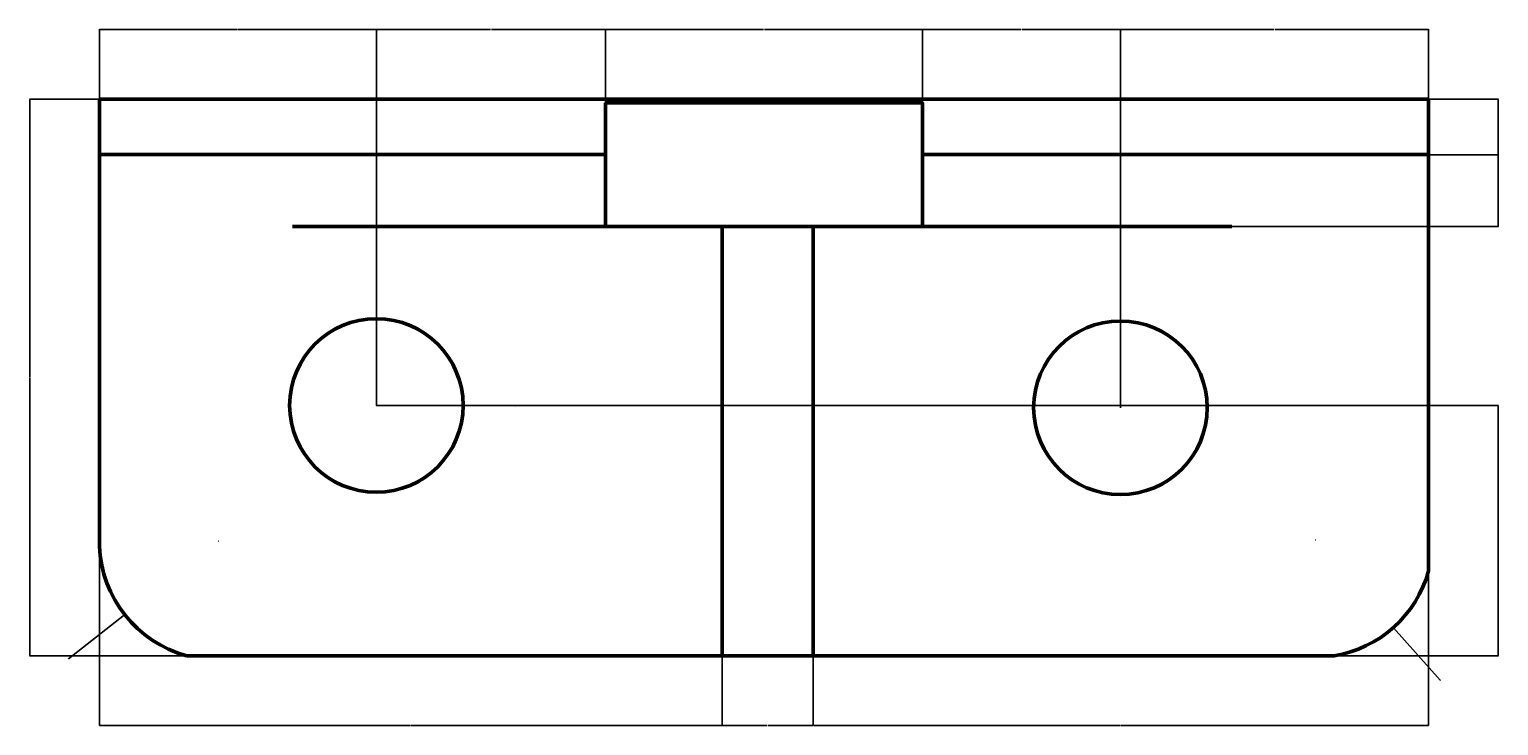
# Model space of a CAD drawing. Units: millimetres. Extents: x 1192 to 5273, y 919 to 2510.
# Tile 2 of 2: x 3955 to 5273, y 1385 to 2010. Entities that reach past the tile are written whole.
import ezdxf

# ---------------------------------------------------------------- set-up
doc = ezdxf.new("R2010")
doc.units = ezdxf.units.MM
doc.layers.add('M-DIMS', color=2, linetype='Continuous', lineweight=18)
doc.layers.add('M-OUTL', color=7, linetype='Continuous', lineweight=50)
doc.styles.get("Standard").update_dxf_attribs({"font": 'arial.ttf'})
doc.dimstyles.get("Standard").update_dxf_attribs({"dimtxt": 0.18, "dimasz": 0.18, "dimexe": 0.18, "dimexo": 0.0625, "dimgap": 0.09, "dimtad": 0, "dimtih": 1, "dimtoh": 1, "dimdec": 4, "dimzin": 0, "dimdsep": 46, "dimtxsty": 'Standard', "dimcen": 0.09, "dimadec": 0, "dimazin": 0, "dimtfac": 1, "dimtdec": 4, "dimtofl": 0, "dimtmove": 0, "dimatfit": 3, "dimfxl": 1, "dimtolj": 1, "dimtzin": 0, "dimarcsym": 0})

# ---------------------------------------------------------------- blocks, each defined once
blk = doc.blocks.new('*D24')
at = {"layer": 'Defpoints', "color": 0, "transparency": 16777216}
for p in [(4017.6, 1545.9), (4576.1, 1447.5), (4576.1, 1385)]:
    blk.add_point(p, dxfattribs=at)
at = {"layer": 'M-DIMS', "color": 0, "lineweight": -2, "transparency": 16777216}
for p, q in [((4017.6, 1545.8), (4017.6, 1384.8)), ((4576.1, 1447.4), (4576.1, 1384.8)), ((4017.8, 1385), (4296.5, 1385)), ((4575.9, 1385), (4297.3, 1385))]:
    blk.add_line(p, q, dxfattribs=at)
at = {"layer": 'M-DIMS', "color": 0, "transparency": 16777216}
for points in [[(4017.8, 1385), (4017.8, 1385), (4017.6, 1385)], [(4575.9, 1385), (4575.9, 1385), (4576.1, 1385)]]:
    blk.add_solid(points, dxfattribs=at)
at = {"layer": 'M-DIMS', "color": 0, "transparency": 16777216, "insert": (4296.9, 1385), "char_height": 0.18, "attachment_point": 5}
blk.add_mtext('\\A1;558.5', dxfattribs=at)
blk = doc.blocks.new('*D25')
at = {"layer": 'Defpoints', "color": 0, "transparency": 16777216}
for p in [(4576.1, 1447.5), (4657.8, 1447.5), (4657.8, 1385)]:
    blk.add_point(p, dxfattribs=at)
at = {"layer": 'M-DIMS', "color": 0, "lineweight": -2, "transparency": 16777216}
for p, q in [((4576.1, 1447.4), (4576.1, 1384.8)), ((4657.8, 1447.4), (4657.8, 1384.8)), ((4576.3, 1385), (4616.6, 1385)), ((4657.6, 1385), (4617.3, 1385))]:
    blk.add_line(p, q, dxfattribs=at)
at = {"layer": 'M-DIMS', "color": 0, "transparency": 16777216}
for points in [[(4576.3, 1385), (4576.3, 1385), (4576.1, 1385)], [(4657.6, 1385), (4657.6, 1385), (4657.8, 1385)]]:
    blk.add_solid(points, dxfattribs=at)
at = {"layer": 'M-DIMS', "color": 0, "transparency": 16777216, "insert": (4616.9, 1385), "char_height": 0.18, "attachment_point": 5}
blk.add_mtext('\\A1;81.65', dxfattribs=at)
blk = doc.blocks.new('*D26')
at = {"layer": 'Defpoints', "color": 0, "transparency": 16777216}
for p in [(5209.8, 1523.7), (4657.8, 1447.5), (5209.8, 1385)]:
    blk.add_point(p, dxfattribs=at)
at = {"layer": 'M-DIMS', "color": 0, "lineweight": -2, "transparency": 16777216}
for p, q in [((5209.8, 1523.6), (5209.8, 1384.8)), ((4657.8, 1447.4), (4657.8, 1384.8)), ((4658, 1385), (4933.5, 1385)), ((5209.6, 1385), (4934.1, 1385))]:
    blk.add_line(p, q, dxfattribs=at)
at = {"layer": 'M-DIMS', "color": 0, "transparency": 16777216}
for points in [[(4658, 1385), (4658, 1385), (4657.8, 1385)], [(5209.6, 1385), (5209.6, 1385), (5209.8, 1385)]]:
    blk.add_solid(points, dxfattribs=at)
at = {"layer": 'M-DIMS', "color": 0, "transparency": 16777216, "insert": (4933.8, 1385), "char_height": 0.18, "attachment_point": 5}
blk.add_mtext('\\A1;552', dxfattribs=at)
blk = doc.blocks.new('*D27')
at = {"layer": 'Defpoints', "color": 0, "transparency": 16777216}
for p in [(4266, 2009.4), (4017.6, 1946.9), (4266, 1672.1)]:
    blk.add_point(p, dxfattribs=at)
at = {"layer": 'M-DIMS', "color": 0, "lineweight": -2, "transparency": 16777216}
for p, q in [((4017.6, 1946.9), (4017.6, 2009.6)), ((4017.8, 2009.4), (4141.4, 2009.4)), ((4265.8, 2009.4), (4142.2, 2009.4)), ((4266, 1672.2), (4266, 2009.6))]:
    blk.add_line(p, q, dxfattribs=at)
at = {"layer": 'M-DIMS', "color": 0, "transparency": 16777216}
for points in [[(4017.8, 2009.4), (4017.8, 2009.3), (4017.6, 2009.4)], [(4265.8, 2009.4), (4265.8, 2009.3), (4266, 2009.4)]]:
    blk.add_solid(points, dxfattribs=at)
at = {"layer": 'M-DIMS', "color": 0, "transparency": 16777216, "insert": (4141.8, 2009.4), "char_height": 0.18, "attachment_point": 5}
blk.add_mtext('\\A1;248.4', dxfattribs=at)
blk = doc.blocks.new('*D28')
at = {"layer": 'Defpoints', "color": 0, "transparency": 16777216}
for p in [(4471.6, 2009.4), (4471.6, 1943.6), (4266, 1672.1)]:
    blk.add_point(p, dxfattribs=at)
at = {"layer": 'M-DIMS', "color": 0, "lineweight": -2, "transparency": 16777216}
for p, q in [((4266, 1672.2), (4266, 2009.6)), ((4266.2, 2009.4), (4368.4, 2009.4)), ((4471.4, 2009.4), (4369.2, 2009.4)), ((4471.6, 1943.7), (4471.6, 2009.6))]:
    blk.add_line(p, q, dxfattribs=at)
at = {"layer": 'M-DIMS', "color": 0, "transparency": 16777216}
for points in [[(4266.2, 2009.4), (4266.2, 2009.3), (4266, 2009.4)], [(4471.4, 2009.4), (4471.4, 2009.3), (4471.6, 2009.4)]]:
    blk.add_solid(points, dxfattribs=at)
at = {"layer": 'M-DIMS', "color": 0, "transparency": 16777216, "insert": (4368.8, 2009.4), "char_height": 0.18, "attachment_point": 5}
blk.add_mtext('\\A1;205.6', dxfattribs=at)
blk = doc.blocks.new('*D29')
at = {"layer": 'Defpoints', "color": 0, "transparency": 16777216}
for p in [(4755.8, 2009.4), (4471.6, 1943.6), (4755.8, 1943.6)]:
    blk.add_point(p, dxfattribs=at)
at = {"layer": 'M-DIMS', "color": 0, "lineweight": -2, "transparency": 16777216}
for p, q in [((4471.6, 1943.7), (4471.6, 2009.6)), ((4471.8, 2009.4), (4613.2, 2009.4)), ((4755.6, 2009.4), (4614.1, 2009.4)), ((4755.8, 1943.7), (4755.8, 2009.6))]:
    blk.add_line(p, q, dxfattribs=at)
at = {"layer": 'M-DIMS', "color": 0, "transparency": 16777216}
for points in [[(4471.8, 2009.4), (4471.8, 2009.3), (4471.6, 2009.4)], [(4755.6, 2009.4), (4755.6, 2009.3), (4755.8, 2009.4)]]:
    blk.add_solid(points, dxfattribs=at)
at = {"layer": 'M-DIMS', "color": 0, "transparency": 16777216, "insert": (4613.7, 2009.4), "char_height": 0.18, "attachment_point": 5}
blk.add_mtext('\\A1;284.16', dxfattribs=at)
blk = doc.blocks.new('*D30')
at = {"layer": 'Defpoints', "color": 0, "transparency": 16777216}
for p in [(4933.3, 2009.4), (4755.8, 1943.6), (4933.3, 1670)]:
    blk.add_point(p, dxfattribs=at)
at = {"layer": 'M-DIMS', "color": 0, "lineweight": -2, "transparency": 16777216}
for p, q in [((4755.8, 1943.7), (4755.8, 2009.6)), ((4755.9, 2009.4), (4844.1, 2009.4)), ((4933.2, 2009.4), (4845, 2009.4)), ((4933.3, 1670.1), (4933.3, 2009.6))]:
    blk.add_line(p, q, dxfattribs=at)
at = {"layer": 'M-DIMS', "color": 0, "transparency": 16777216}
for points in [[(4755.9, 2009.4), (4755.9, 2009.3), (4755.8, 2009.4)], [(4933.2, 2009.4), (4933.2, 2009.3), (4933.3, 2009.4)]]:
    blk.add_solid(points, dxfattribs=at)
at = {"layer": 'M-DIMS', "color": 0, "transparency": 16777216, "insert": (4844.5, 2009.4), "char_height": 0.18, "attachment_point": 5}
blk.add_mtext('\\A1;177.57', dxfattribs=at)
blk = doc.blocks.new('*D31')
at = {"layer": 'Defpoints', "color": 0, "transparency": 16777216}
for p in [(5209.8, 2009.4), (5209.8, 1946.9), (4933.3, 1670)]:
    blk.add_point(p, dxfattribs=at)
at = {"layer": 'M-DIMS', "color": 0, "lineweight": -2, "transparency": 16777216}
for p, q in [((4933.3, 1670.1), (4933.3, 2009.6)), ((4933.5, 2009.4), (5071.1, 2009.4)), ((5209.6, 2009.4), (5072, 2009.4)), ((5209.8, 1946.9), (5209.8, 2009.6))]:
    blk.add_line(p, q, dxfattribs=at)
at = {"layer": 'M-DIMS', "color": 0, "transparency": 16777216}
for points in [[(4933.5, 2009.4), (4933.5, 2009.3), (4933.3, 2009.4)], [(5209.6, 2009.4), (5209.6, 2009.3), (5209.8, 2009.4)]]:
    blk.add_solid(points, dxfattribs=at)
at = {"layer": 'M-DIMS', "color": 0, "transparency": 16777216, "insert": (5071.5, 2009.4), "char_height": 0.18, "attachment_point": 5}
blk.add_mtext('\\A1;276.43', dxfattribs=at)
blk = doc.blocks.new('*D32')
at = {"layer": 'Defpoints', "color": 0, "transparency": 16777216}
for p in [(4017.6, 1946.9), (3955.1, 1447.5), (4095.6, 1447.5)]:
    blk.add_point(p, dxfattribs=at)
at = {"layer": 'M-DIMS', "color": 0, "lineweight": -2, "transparency": 16777216}
for p, q in [((4017.5, 1946.9), (3954.9, 1946.9)), ((3955.1, 1946.7), (3955.1, 1697.4)), ((3955.1, 1447.7), (3955.1, 1697)), ((4095.5, 1447.5), (3954.9, 1447.5))]:
    blk.add_line(p, q, dxfattribs=at)
at = {"layer": 'M-DIMS', "color": 0, "transparency": 16777216}
for points in [[(3955.1, 1946.7), (3955.1, 1946.7), (3955.1, 1946.9)], [(3955.1, 1447.7), (3955.1, 1447.7), (3955.1, 1447.5)]]:
    blk.add_solid(points, dxfattribs=at)
at = {"layer": 'M-DIMS', "color": 0, "transparency": 16777216, "insert": (3955.1, 1697.2), "char_height": 0.18, "attachment_point": 5}
blk.add_mtext('\\A1;499.4', dxfattribs=at)
blk = doc.blocks.new('*D33')
at = {"layer": 'Defpoints', "color": 0, "transparency": 16777216}
for p in [(4266, 1672.1), (5272.3, 1672.1), (4095.6, 1447.5)]:
    blk.add_point(p, dxfattribs=at)
at = {"layer": 'M-DIMS', "color": 0, "lineweight": -2, "transparency": 16777216}
for p, q in [((4266.1, 1672.1), (5272.4, 1672.1)), ((5272.3, 1671.9), (5272.3, 1560)), ((5272.3, 1447.7), (5272.3, 1559.6)), ((4095.6, 1447.5), (5272.4, 1447.5))]:
    blk.add_line(p, q, dxfattribs=at)
at = {"layer": 'M-DIMS', "color": 0, "transparency": 16777216}
for points in [[(5272.2, 1671.9), (5272.3, 1671.9), (5272.3, 1672.1)], [(5272.2, 1447.7), (5272.3, 1447.7), (5272.3, 1447.5)]]:
    blk.add_solid(points, dxfattribs=at)
at = {"layer": 'M-DIMS', "color": 0, "transparency": 16777216, "insert": (5272.3, 1559.8), "char_height": 0.18, "attachment_point": 5}
blk.add_mtext('\\A1;224.6', dxfattribs=at)
blk = doc.blocks.new('*D34')
at = {"layer": 'Defpoints', "color": 0, "transparency": 16777216}
for p in [(5209.8, 1946.9), (5209.8, 1897.1), (5272.3, 1897.1)]:
    blk.add_point(p, dxfattribs=at)
at = {"layer": 'M-DIMS', "color": 0, "lineweight": -2, "transparency": 16777216}
for p, q in [((5209.8, 1946.9), (5272.4, 1946.9)), ((5272.3, 1946.7), (5272.3, 1922.2)), ((5272.3, 1897.3), (5272.3, 1921.8)), ((5209.8, 1897.1), (5272.4, 1897.1))]:
    blk.add_line(p, q, dxfattribs=at)
at = {"layer": 'M-DIMS', "color": 0, "transparency": 16777216}
for points in [[(5272.2, 1946.7), (5272.3, 1946.7), (5272.3, 1946.9)], [(5272.2, 1897.3), (5272.3, 1897.3), (5272.3, 1897.1)]]:
    blk.add_solid(points, dxfattribs=at)
at = {"layer": 'M-DIMS', "color": 0, "transparency": 16777216, "insert": (5272.3, 1922), "char_height": 0.18, "attachment_point": 5}
blk.add_mtext('\\A1;49.73', dxfattribs=at)
blk = doc.blocks.new('*D35')
at = {"layer": 'Defpoints', "color": 0, "transparency": 16777216}
for p in [(5209.8, 1897.1), (4755.8, 1832.6), (5272.3, 1832.6)]:
    blk.add_point(p, dxfattribs=at)
at = {"layer": 'M-DIMS', "color": 0, "lineweight": -2, "transparency": 16777216}
for p, q in [((5209.8, 1897.1), (5272.4, 1897.1)), ((5272.3, 1897), (5272.3, 1865.1)), ((5272.3, 1832.8), (5272.3, 1864.7)), ((4755.8, 1832.6), (5272.4, 1832.6))]:
    blk.add_line(p, q, dxfattribs=at)
at = {"layer": 'M-DIMS', "color": 0, "transparency": 16777216}
for points in [[(5272.2, 1897), (5272.3, 1897), (5272.3, 1897.1)], [(5272.2, 1832.8), (5272.3, 1832.8), (5272.3, 1832.6)]]:
    blk.add_solid(points, dxfattribs=at)
at = {"layer": 'M-DIMS', "color": 0, "transparency": 16777216, "insert": (5272.3, 1864.9), "char_height": 0.18, "attachment_point": 5}
blk.add_mtext('\\A1;64.51', dxfattribs=at)
blk = doc.blocks.new('*D40')
at = {"layer": 'Defpoints', "color": 0, "transparency": 16777216}
for p in [(4188.2, 1672.2), (4343.8, 1672)]:
    blk.add_point(p, dxfattribs=at)
at = {"layer": 'M-DIMS', "color": 0, "lineweight": -2, "transparency": 16777216}
for p, q in [((4265.9, 1672.1), (4266.1, 1672.1)), ((4266, 1672), (4266, 1672.2)), ((4390.5, 1671.9), (4344, 1672))]:
    blk.add_line(p, q, dxfattribs=at)
at = {"layer": 'M-DIMS', "color": 0, "transparency": 16777216}
blk.add_solid([(4344, 1672), (4344, 1672), (4343.8, 1672)], dxfattribs=at)
at = {"layer": 'M-DIMS', "color": 0, "transparency": 16777216, "insert": (4391.3, 1671.9), "char_height": 0.18, "attachment_point": 5}
blk.add_mtext('\\A1;2X ∅155.67', dxfattribs=at)
blk = doc.blocks.new('*D41')
at = {"layer": 'Defpoints', "color": 0, "transparency": 16777216}
for p in [(4124.3, 1550.4), (4040.4, 1484.3)]:
    blk.add_point(p, dxfattribs=at)
at = {"layer": 'M-DIMS', "color": 0, "lineweight": -2, "transparency": 16777216}
for p, q in [((4124.2, 1550.4), (4124.4, 1550.4)), ((4124.3, 1550.3), (4124.3, 1550.4)), ((3990, 1444.7), (4040.2, 1484.2)), ((3989.9, 1444.7), (3990, 1444.7))]:
    blk.add_line(p, q, dxfattribs=at)
at = {"layer": 'M-DIMS', "color": 0, "transparency": 16777216}
blk.add_solid([(4040.2, 1484.2), (4040.3, 1484.2), (4040.4, 1484.3)], dxfattribs=at)
at = {"layer": 'M-DIMS', "color": 0, "transparency": 16777216, "insert": (3989.3, 1444.7), "char_height": 0.18, "attachment_point": 5}
blk.add_mtext('\\A1;R106.79', dxfattribs=at)
blk = doc.blocks.new('*D42')
at = {"layer": 'Defpoints', "color": 0, "transparency": 16777216}
for p in [(5108.1, 1551.5), (5178.2, 1472.8)]:
    blk.add_point(p, dxfattribs=at)
at = {"layer": 'M-DIMS', "color": 0, "lineweight": -2, "transparency": 16777216}
for p, q in [((5108.1, 1551.4), (5108.1, 1551.6)), ((5108.1, 1551.5), (5108.2, 1551.5)), ((5220.2, 1425.6), (5178.3, 1472.7)), ((5220.4, 1425.6), (5220.2, 1425.6))]:
    blk.add_line(p, q, dxfattribs=at)
at = {"layer": 'M-DIMS', "color": 0, "transparency": 16777216}
blk.add_solid([(5178.3, 1472.7), (5178.3, 1472.6), (5178.2, 1472.8)], dxfattribs=at)
at = {"layer": 'M-DIMS', "color": 0, "transparency": 16777216, "insert": (5220.9, 1425.6), "char_height": 0.18, "attachment_point": 5}
blk.add_mtext('\\A1;R105.36', dxfattribs=at)

msp = doc.modelspace()

# ---------------------------------------------------------------- linework, layer by layer
at = {"layer": 'M-OUTL'}
for p, q in [((4017.602, 1946.875), (5209.763, 1946.875)), ((4576.122, 1946.875), (4576.122, 1943.611)), ((4657.776, 1946.875), (4657.776, 1943.611)), ((4017.602, 1897.148), (4471.603, 1897.148)), ((4755.762, 1897.148), (5209.763, 1897.148)), ((4471.603, 1832.639), (4190.711, 1832.639)), ((4576.122, 1832.639), (4576.122, 1447.499)), ((4657.776, 1832.639), (4657.776, 1447.499)), ((4755.762, 1832.639), (5033.389, 1832.639)), ((4095.57, 1447.499), (5124.948, 1447.499))]:
    msp.add_line(p, q, dxfattribs=at)
for points in [[(4017.602, 1545.887), (4017.602, 1946.875)], [(5209.763, 1946.875), (5209.763, 1523.657)]]:
    msp.add_lwpolyline(points, dxfattribs=at)
msp.add_lwpolyline([(4471.603, 1943.611), (4755.762, 1943.611), (4755.762, 1832.639), (4471.603, 1832.639)], close=True, dxfattribs=at)
for centre in [(4266.004, 1672.109), (4933.332, 1670.045), (4933.332, 1670.045)]:
    msp.add_circle(centre, 77.834, dxfattribs=at)
for centre, radius, start, end in [((4124.298, 1550.351), 106.788, 182.395749, 254.394373), ((5108.149, 1551.516), 105.364, 279.174107, 344.668418)]:
    msp.add_arc(centre, radius, start, end, dxfattribs=at)

# ---------------------------------------------------------------- dimensions: what is measured, and where the dimension line sits
at = {"layer": 'M-DIMS'}
for base, p1, p2, override, picture, middle in [((4266.004, 2009.375), (4017.602, 1946.875), (4266.004, 1672.109), {"dimdec": 1, "dimlfac": 1, "dimrnd": 0, "dimzin": 0, "dimdsep": 46, "dimlunit": 2}, '*D27', (4141.803, 2009.375)), ((4471.603, 2009.375), (4266.004, 1672.109), (4471.603, 1943.611), {"dimdec": 1, "dimlfac": 1, "dimrnd": 0, "dimzin": 0, "dimdsep": 46, "dimlunit": 2}, '*D28', (4368.804, 2009.375)), ((4755.762, 2009.375), (4471.603, 1943.611), (4755.762, 1943.611), {"dimdec": 2, "dimlfac": 1, "dimrnd": 0, "dimzin": 0, "dimdsep": 46, "dimlunit": 2}, '*D29', (4613.683, 2009.375)), ((4933.332, 2009.375), (4755.762, 1943.611), (4933.332, 1670.045), {"dimdec": 2, "dimlfac": 1, "dimrnd": 0, "dimzin": 0, "dimdsep": 46, "dimlunit": 2}, '*D30', (4844.547, 2009.375)), ((5209.763, 2009.375), (4933.332, 1670.045), (5209.763, 1946.875), {"dimdec": 2, "dimlfac": 1, "dimrnd": 0, "dimzin": 0, "dimdsep": 46, "dimlunit": 2}, '*D31', (5071.548, 2009.375)), ((4576.122, 1384.999), (4017.602, 1545.887), (4576.122, 1447.499), {"dimdec": 1, "dimlfac": 1, "dimrnd": 0, "dimzin": 0, "dimdsep": 46, "dimlunit": 2}, '*D24', (4296.862, 1384.999)), ((5209.763, 1384.999), (4657.776, 1447.499), (5209.763, 1523.657), {"dimdec": 0, "dimlfac": 1, "dimrnd": 0, "dimzin": 0, "dimdsep": 46, "dimlunit": 2}, '*D26', (4933.77, 1384.999)), ((4657.776, 1384.999), (4576.122, 1447.499), (4657.776, 1447.499), {"dimdec": 2, "dimlfac": 1, "dimrnd": 0, "dimzin": 0, "dimdsep": 46, "dimlunit": 2}, '*D25', (4616.949, 1384.999))]:
    dim = msp.add_linear_dim(base=base, p1=p1, p2=p2, dimstyle='Standard', override=override, dxfattribs=at)
    dim.commit()
    dim.dimension.update_dxf_attribs({"geometry": picture, "text_midpoint": middle})
for base, p1, p2, override, picture, middle in [((3955.103, 1447.499), (4017.602, 1946.875), (4095.57, 1447.499), {"dimdec": 1, "dimlfac": 1, "dimrnd": 0, "dimzin": 0, "dimdsep": 46, "dimlunit": 2}, '*D32', (3955.103, 1697.187)), ((5272.263, 1897.148), (5209.763, 1946.875), (5209.763, 1897.148), {"dimdec": 2, "dimlfac": 1, "dimrnd": 0, "dimzin": 0, "dimdsep": 46, "dimlunit": 2}, '*D34', (5272.263, 1922.012)), ((5272.263, 1832.639), (5209.763, 1897.148), (4755.762, 1832.639), {"dimdec": 2, "dimlfac": 1, "dimrnd": 0, "dimzin": 0, "dimdsep": 46, "dimlunit": 2}, '*D35', (5272.263, 1864.894)), ((5272.263, 1672.109), (4095.57, 1447.499), (4266.004, 1672.109), {"dimdec": 1, "dimlfac": 1, "dimrnd": 0, "dimzin": 0, "dimdsep": 46, "dimlunit": 2}, '*D33', (5272.263, 1559.804))]:
    dim = msp.add_linear_dim(base=base, p1=p1, p2=p2, angle=90, dimstyle='Standard', override=override, dxfattribs=at)
    dim.commit()
    dim.dimension.update_dxf_attribs({"geometry": picture, "text_midpoint": middle})
dim = msp.add_diameter_dim_2p(p1=(4188.17, 1672.22), p2=(4343.839, 1671.999), text='2X <>', dimstyle='Standard', override={"dimdec": 2, "dimlfac": 1, "dimrnd": 0, "dimzin": 0, "dimdsep": 46, "dimlunit": 2}, dxfattribs=at)
dim.commit()
dim.dimension.update_dxf_attribs({"geometry": '*D40', "text_midpoint": (4390.539, 1671.932), "dimtype": 163})
for center, mpoint, picture, middle in [((4124.298, 1550.351), (4040.385, 1484.303), '*D41', (3989.307, 1444.674)), ((5108.149, 1551.516), (5178.182, 1472.795), '*D42', (5220.932, 1425.563))]:
    dim = msp.add_radius_dim(center=center, mpoint=mpoint, dimstyle='Standard', override={"dimdec": 2, "dimlfac": 1, "dimrnd": 0, "dimzin": 0, "dimdsep": 46, "dimlunit": 2}, dxfattribs=at)
    dim.commit()
    dim.dimension.update_dxf_attribs({"geometry": picture, "text_midpoint": middle, "dimtype": 164})

doc.saveas('drawing.dxf')
